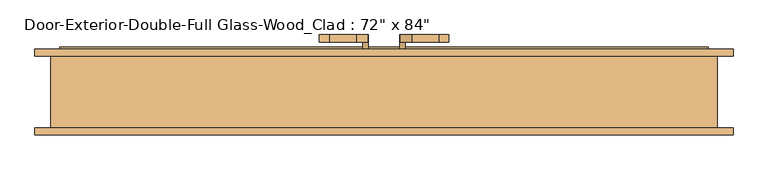
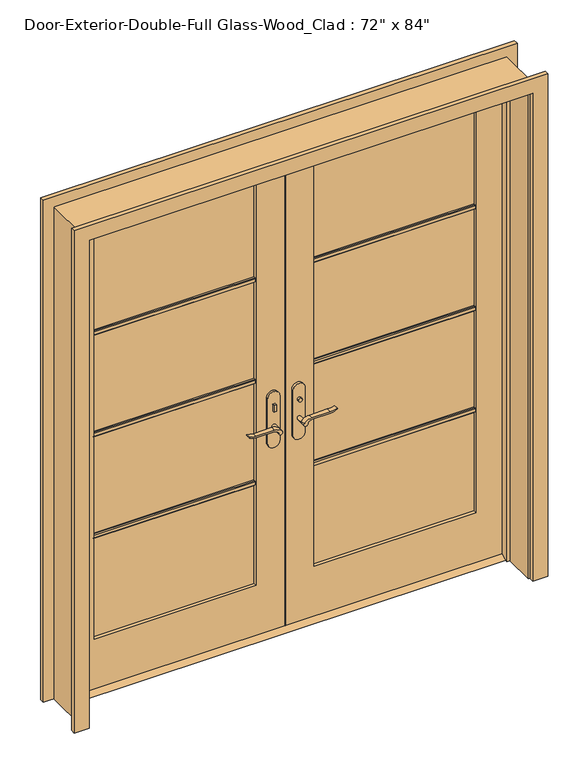
"""IFC4 building model written with IfcOpenShell, lengths in millimetres: door geometry."""

from ifc_helpers import new_model, si_unit, point, frame, frame_2d, origin, place, context, project, spatial, polyline, circle_curve, trimmed, segment, composite_curve, outline, extrude, faceted_brep, source, transform, mapped, element, save


def door_06d7e188(model_context):
    return source(origin(), model_context, "Body", "SolidModel", [
        extrude(outline(polyline([(63.5, 12.7), (98.425, 12.7), (123.825, 0.0), (38.1, 0.0), (63.5, 12.7)])), frame((-914.4, 0.0, 0.0), z_axis=(1.0, 0.0, 0.0), x_axis=(0.0, 1.0, 0.0)), (0.0, 0.0, 1.0), 1828.8),
        extrude(outline(polyline([(-47.4019111, 43.5), (-57.4019111, 43.5), (-57.4019111, 53.5), (-47.4019111, 53.5), (-47.4019111, 43.5)])), frame((0.0, 0.0, 981.9), z_axis=(0.0, 0.0, 1.0), x_axis=(1.0, 0.0, 0.0)), (0.0, 0.0, 1.0), 30.0),
        extrude(outline(composite_curve([segment(trimmed(circle_curve(frame_2d((996.9, -52.4019111)), 8.0), [point((996.9, -60.4019111))], [point((996.9, -44.4019111))], False, "CARTESIAN"), True, "CONTINUOUS"), segment(trimmed(circle_curve(frame_2d((996.9, -52.4019111)), 8.0), [point((996.9, -44.4019111))], [point((996.9, -60.4019111))], False, "CARTESIAN"), True, "CONTINUOUS")], self_intersect=False)), frame((0.0, 108.425, 0.0), z_axis=(0.0, 1.0, 0.0), x_axis=(0.0, 0.0, 1.0)), (0.0, 0.0, 1.0), 10.0),
        extrude(outline(composite_curve([segment(trimmed(circle_curve(frame_2d((897.1555521, -76.0694241)), 37.2832219), [point((919.0523287, -45.8937749))], [point((934.4, -77.7693445))], False, "CARTESIAN"), True, "CONTINUOUS"), segment(polyline([(934.4, -77.7693445), (934.4, -154.045502)]), True, "CONTINUOUS"), segment(trimmed(circle_curve(frame_2d((1017.6850638, -153.9791202)), 83.2850902), [point((934.4, -154.045502))], [point((939.4, -182.4019111))], True, "CARTESIAN"), True, "CONTINUOUS"), segment(polyline([(939.4, -182.4019111), (936.6135558, -182.4019111)]), True, "CONTINUOUS"), segment(trimmed(circle_curve(frame_2d((986.6709207, -150.4622499)), 59.3791355), [point((936.6135558, -182.4019111))], [point((927.4, -154.045502))], False, "CARTESIAN"), True, "CONTINUOUS"), segment(polyline([(927.4, -154.045502), (927.4, -77.7881013)]), True, "CONTINUOUS"), segment(trimmed(circle_curve(frame_2d((909.2738613, -77.7881013)), 18.1261387), [point((927.4, -77.7881013))], [point((914.4, -60.4019111))], True, "CARTESIAN"), True, "CONTINUOUS"), segment(trimmed(circle_curve(frame_2d((914.4, -52.4019111)), 8.0), [point((914.4, -60.4019111))], [point((919.0523287, -45.8937749))], False, "CARTESIAN"), True, "CONTINUOUS")], self_intersect=False)), frame((0.0, 3.5, 0.0), z_axis=(0.0, 1.0, 0.0), x_axis=(0.0, 0.0, 1.0)), (0.0, 0.0, 1.0), 20.0),
        extrude(outline(composite_curve([segment(trimmed(circle_curve(frame_2d((914.4, -52.4019111)), 8.0), [point((914.3999903, -60.4019111))], [point((919.0523287, -45.8937749))], False, "CARTESIAN"), True, "CONTINUOUS"), segment(trimmed(circle_curve(frame_2d((897.1555521, -76.0694241)), 37.2832219), [point((919.0523287, -45.8937749))], [point((934.4, -77.7693445))], False, "CARTESIAN"), True, "CONTINUOUS"), segment(polyline([(934.4, -77.7693445), (934.4, -154.045502)]), True, "CONTINUOUS"), segment(trimmed(circle_curve(frame_2d((1017.6850638, -153.9791202)), 83.2850902), [point((934.4, -154.045502))], [point((939.4, -182.4019111))], True, "CARTESIAN"), True, "CONTINUOUS"), segment(polyline([(939.4, -182.4019111), (936.6135558, -182.4019111)]), True, "CONTINUOUS"), segment(trimmed(circle_curve(frame_2d((986.6709207, -150.4622499)), 59.3791355), [point((936.6135558, -182.4019111))], [point((927.4, -154.045502))], False, "CARTESIAN"), True, "CONTINUOUS"), segment(polyline([(927.4, -154.045502), (927.4, -77.788099)]), True, "CONTINUOUS"), segment(trimmed(circle_curve(frame_2d((909.2738682, -77.788099)), 18.1261318), [point((927.4, -77.788099))], [point((914.3999903, -60.4019111))], True, "CARTESIAN"), True, "CONTINUOUS")], self_intersect=False)), frame((0.0, 138.425, 0.0), z_axis=(0.0, 1.0, 0.0), x_axis=(0.0, 0.0, 1.0)), (0.0, 0.0, 1.0), 20.0),
        extrude(outline(composite_curve([segment(trimmed(circle_curve(frame_2d((914.4, -52.4019111)), 8.0), [point((914.4, -60.4019111))], [point((914.4, -44.4019111))], False, "CARTESIAN"), True, "CONTINUOUS"), segment(trimmed(circle_curve(frame_2d((914.4, -52.4019111)), 8.0), [point((914.4, -44.4019111))], [point((914.4, -60.4019111))], False, "CARTESIAN"), True, "CONTINUOUS")], self_intersect=False)), frame((0.0, 23.5, 0.0), z_axis=(0.0, 1.0, 0.0), x_axis=(0.0, 0.0, 1.0)), (0.0, 0.0, 1.0), 30.0),
        extrude(outline(composite_curve([segment(trimmed(circle_curve(frame_2d((914.4, -52.4019111)), 8.0), [point((914.4, -60.4019111))], [point((914.4, -44.4019111))], False, "CARTESIAN"), True, "CONTINUOUS"), segment(trimmed(circle_curve(frame_2d((914.4, -52.4019111)), 8.0), [point((914.4, -44.4019111))], [point((914.4, -60.4019111))], False, "CARTESIAN"), True, "CONTINUOUS")], self_intersect=False)), frame((0.0, 108.425, 0.0), z_axis=(0.0, 1.0, 0.0), x_axis=(0.0, 0.0, 1.0)), (0.0, 0.0, 1.0), 30.0),
        extrude(outline(composite_curve([segment(polyline([(844.4, -27.4019111), (1039.4, -27.4019111)]), True, "CONTINUOUS"), segment(trimmed(circle_curve(frame_2d((1039.4, -52.4019111)), 25.0), [point((1039.4, -27.4019111))], [point((1039.4, -77.4019111))], False, "CARTESIAN"), True, "CONTINUOUS"), segment(polyline([(1039.4, -77.4019111), (844.4, -77.4019111)]), True, "CONTINUOUS"), segment(trimmed(circle_curve(frame_2d((844.4, -52.4019111)), 25.0), [point((844.4, -77.4019111))], [point((844.4, -27.4019111))], False, "CARTESIAN"), True, "CONTINUOUS")], self_intersect=False)), frame((0.0, 53.5, 0.0), z_axis=(0.0, 1.0, 0.0), x_axis=(0.0, 0.0, 1.0)), (0.0, 0.0, 1.0), 10.0),
        extrude(outline(composite_curve([segment(polyline([(844.4, -27.4019111), (1039.4, -27.4019111)]), True, "CONTINUOUS"), segment(trimmed(circle_curve(frame_2d((1039.4, -52.4019111)), 25.0), [point((1039.4, -27.4019111))], [point((1039.4, -77.4019111))], False, "CARTESIAN"), True, "CONTINUOUS"), segment(polyline([(1039.4, -77.4019111), (844.4, -77.4019111)]), True, "CONTINUOUS"), segment(trimmed(circle_curve(frame_2d((844.4, -52.4019111)), 25.0), [point((844.4, -77.4019111))], [point((844.4, -27.4019111))], False, "CARTESIAN"), True, "CONTINUOUS")], self_intersect=False)), frame((0.0, 98.425, 0.0), z_axis=(0.0, 1.0, 0.0), x_axis=(0.0, 0.0, 1.0)), (0.0, 0.0, 1.0), 10.0),
        extrude(outline(polyline([(47.3875, 118.425), (57.3875, 118.425), (57.3875, 108.425), (47.3875, 108.425), (47.3875, 118.425)])), frame((0.0, 0.0, 981.9), z_axis=(0.0, 0.0, 1.0), x_axis=(1.0, 0.0, 0.0)), (0.0, 0.0, 1.0), 30.0),
        extrude(outline(composite_curve([segment(trimmed(circle_curve(frame_2d((996.9, 52.3875)), 8.0), [point((996.9, 60.3875))], [point((996.9, 44.3875))], False, "CARTESIAN"), True, "CONTINUOUS"), segment(trimmed(circle_curve(frame_2d((996.9, 52.3875)), 8.0), [point((996.9, 44.3875))], [point((996.9, 60.3875))], False, "CARTESIAN"), True, "CONTINUOUS")], self_intersect=False)), frame((0.0, 43.5, 0.0), z_axis=(0.0, 1.0, 0.0), x_axis=(0.0, 0.0, 1.0)), (0.0, 0.0, 1.0), 10.0),
        extrude(outline(composite_curve([segment(trimmed(circle_curve(frame_2d((914.4, 52.3875)), 8.0), [point((919.0523287, 45.8793637))], [point((914.4, 60.3875))], False, "CARTESIAN"), True, "CONTINUOUS"), segment(trimmed(circle_curve(frame_2d((909.2738613, 77.7736901)), 18.1261387), [point((914.4, 60.3875))], [point((927.4, 77.7736901))], True, "CARTESIAN"), True, "CONTINUOUS"), segment(polyline([(927.4, 77.7736901), (927.4, 154.0310909)]), True, "CONTINUOUS"), segment(trimmed(circle_curve(frame_2d((986.6709207, 150.4478388)), 59.3791355), [point((927.4, 154.0310909))], [point((936.6135558, 182.3875))], False, "CARTESIAN"), True, "CONTINUOUS"), segment(polyline([(936.6135558, 182.3875), (939.4, 182.3875)]), True, "CONTINUOUS"), segment(trimmed(circle_curve(frame_2d((1017.6850638, 153.9647091)), 83.2850902), [point((939.4, 182.3875))], [point((934.4, 154.0310909))], True, "CARTESIAN"), True, "CONTINUOUS"), segment(polyline([(934.4, 154.0310909), (934.4, 77.7549333)]), True, "CONTINUOUS"), segment(trimmed(circle_curve(frame_2d((897.1555521, 76.0550129)), 37.2832219), [point((934.4, 77.7549333))], [point((919.0523287, 45.8793637))], False, "CARTESIAN"), True, "CONTINUOUS")], self_intersect=False)), frame((0.0, 138.425, 0.0), z_axis=(0.0, 1.0, 0.0), x_axis=(0.0, 0.0, 1.0)), (0.0, 0.0, 1.0), 20.0),
        extrude(outline(composite_curve([segment(trimmed(circle_curve(frame_2d((909.2738682, 77.7736878)), 18.1261318), [point((914.3999903, 60.3875))], [point((927.4, 77.7736878))], True, "CARTESIAN"), True, "CONTINUOUS"), segment(polyline([(927.4, 77.7736878), (927.4, 154.0310909)]), True, "CONTINUOUS"), segment(trimmed(circle_curve(frame_2d((986.6709207, 150.4478388)), 59.3791355), [point((927.4, 154.0310909))], [point((936.6135558, 182.3875))], False, "CARTESIAN"), True, "CONTINUOUS"), segment(polyline([(936.6135558, 182.3875), (939.4, 182.3875)]), True, "CONTINUOUS"), segment(trimmed(circle_curve(frame_2d((1017.6850638, 153.9647091)), 83.2850902), [point((939.4, 182.3875))], [point((934.4, 154.0310909))], True, "CARTESIAN"), True, "CONTINUOUS"), segment(polyline([(934.4, 154.0310909), (934.4, 77.7549333)]), True, "CONTINUOUS"), segment(trimmed(circle_curve(frame_2d((897.1555521, 76.0550129)), 37.2832219), [point((934.4, 77.7549333))], [point((919.0523287, 45.8793637))], False, "CARTESIAN"), True, "CONTINUOUS"), segment(trimmed(circle_curve(frame_2d((914.4, 52.3875)), 8.0), [point((919.0523287, 45.8793637))], [point((914.3999903, 60.3875))], False, "CARTESIAN"), True, "CONTINUOUS")], self_intersect=False)), frame((0.0, 3.5, 0.0), z_axis=(0.0, 1.0, 0.0), x_axis=(0.0, 0.0, 1.0)), (0.0, 0.0, 1.0), 20.0),
        extrude(outline(composite_curve([segment(trimmed(circle_curve(frame_2d((914.4, 52.3875)), 8.0), [point((914.4, 60.3875))], [point((914.4, 44.3875))], False, "CARTESIAN"), True, "CONTINUOUS"), segment(trimmed(circle_curve(frame_2d((914.4, 52.3875)), 8.0), [point((914.4, 44.3875))], [point((914.4, 60.3875))], False, "CARTESIAN"), True, "CONTINUOUS")], self_intersect=False)), frame((0.0, 108.425, 0.0), z_axis=(0.0, 1.0, 0.0), x_axis=(0.0, 0.0, 1.0)), (0.0, 0.0, 1.0), 30.0),
        extrude(outline(composite_curve([segment(trimmed(circle_curve(frame_2d((914.4, 52.3875)), 8.0), [point((914.4, 60.3875))], [point((914.4, 44.3875))], False, "CARTESIAN"), True, "CONTINUOUS"), segment(trimmed(circle_curve(frame_2d((914.4, 52.3875)), 8.0), [point((914.4, 44.3875))], [point((914.4, 60.3875))], False, "CARTESIAN"), True, "CONTINUOUS")], self_intersect=False)), frame((0.0, 23.5, 0.0), z_axis=(0.0, 1.0, 0.0), x_axis=(0.0, 0.0, 1.0)), (0.0, 0.0, 1.0), 30.0),
        extrude(outline(composite_curve([segment(trimmed(circle_curve(frame_2d((844.4, 52.3875)), 25.0), [point((844.4, 27.3875))], [point((844.4, 77.3875))], False, "CARTESIAN"), True, "CONTINUOUS"), segment(polyline([(844.4, 77.3875), (1039.4, 77.3875)]), True, "CONTINUOUS"), segment(trimmed(circle_curve(frame_2d((1039.4, 52.3875)), 25.0), [point((1039.4, 77.3875))], [point((1039.4, 27.3875))], False, "CARTESIAN"), True, "CONTINUOUS"), segment(polyline([(1039.4, 27.3875), (844.4, 27.3875)]), True, "CONTINUOUS")], self_intersect=False)), frame((0.0, 98.425, 0.0), z_axis=(0.0, 1.0, 0.0), x_axis=(0.0, 0.0, 1.0)), (0.0, 0.0, 1.0), 10.0),
        extrude(outline(composite_curve([segment(trimmed(circle_curve(frame_2d((844.4, 52.3875)), 25.0), [point((844.4, 27.3875))], [point((844.4, 77.3875))], False, "CARTESIAN"), True, "CONTINUOUS"), segment(polyline([(844.4, 77.3875), (1039.4, 77.3875)]), True, "CONTINUOUS"), segment(trimmed(circle_curve(frame_2d((1039.4, 52.3875)), 25.0), [point((1039.4, 77.3875))], [point((1039.4, 27.3875))], False, "CARTESIAN"), True, "CONTINUOUS"), segment(polyline([(1039.4, 27.3875), (844.4, 27.3875)]), True, "CONTINUOUS")], self_intersect=False)), frame((0.0, 53.5, 0.0), z_axis=(0.0, 1.0, 0.0), x_axis=(0.0, 0.0, 1.0)), (0.0, 0.0, 1.0), 10.0),
        extrude(outline(polyline([(77.47, 1578.371875), (77.47, 1559.321875), (71.12, 1559.321875), (67.945, 1562.496875), (67.945, 1575.196875), (71.12, 1578.371875), (77.47, 1578.371875)])), frame((120.65, 0.0, 0.0), z_axis=(1.0, 0.0, 0.0), x_axis=(0.0, 1.0, 0.0)), (0.0, 0.0, 1.0), 673.1),
        extrude(outline(polyline([(77.47, 1132.68125), (77.47, 1113.63125), (71.12, 1113.63125), (67.945, 1116.80625), (67.945, 1129.50625), (71.12, 1132.68125), (77.47, 1132.68125)])), frame((120.65, 0.0, 0.0), z_axis=(1.0, 0.0, 0.0), x_axis=(0.0, 1.0, 0.0)), (0.0, 0.0, 1.0), 673.1),
        extrude(outline(polyline([(77.47, 686.990625), (77.47, 667.940625), (71.12, 667.940625), (67.945, 671.115625), (67.945, 683.815625), (71.12, 686.990625), (77.47, 686.990625)])), frame((120.65, 0.0, 0.0), z_axis=(1.0, 0.0, 0.0), x_axis=(0.0, 1.0, 0.0)), (0.0, 0.0, 1.0), 673.1),
        extrude(outline(polyline([(84.455, 1578.371875), (90.805, 1578.371875), (93.98, 1575.196875), (93.98, 1562.496875), (90.805, 1559.321875), (84.455, 1559.321875), (84.455, 1578.371875)])), frame((-793.75, 0.0, 0.0), z_axis=(1.0, 0.0, 0.0), x_axis=(0.0, 1.0, 0.0)), (0.0, 0.0, 1.0), 673.1),
        extrude(outline(polyline([(84.455, 1132.68125), (90.805, 1132.68125), (93.98, 1129.50625), (93.98, 1116.80625), (90.805, 1113.63125), (84.455, 1113.63125), (84.455, 1132.68125)])), frame((-793.75, 0.0, 0.0), z_axis=(1.0, 0.0, 0.0), x_axis=(0.0, 1.0, 0.0)), (0.0, 0.0, 1.0), 673.1),
        extrude(outline(polyline([(84.455, 686.990625), (90.805, 686.990625), (93.98, 683.815625), (93.98, 671.115625), (90.805, 667.940625), (84.455, 667.940625), (84.455, 686.990625)])), frame((-793.75, 0.0, 0.0), z_axis=(1.0, 0.0, 0.0), x_axis=(0.0, 1.0, 0.0)), (0.0, 0.0, 1.0), 673.1),
        extrude(outline(polyline([(84.455, 1578.371875), (90.805, 1578.371875), (93.98, 1575.196875), (93.98, 1562.496875), (90.805, 1559.321875), (84.455, 1559.321875), (84.455, 1578.371875)])), frame((120.65, 0.0, 0.0), z_axis=(1.0, 0.0, 0.0), x_axis=(0.0, 1.0, 0.0)), (0.0, 0.0, 1.0), 673.1),
        extrude(outline(polyline([(84.455, 1132.68125), (90.805, 1132.68125), (93.98, 1129.50625), (93.98, 1116.80625), (90.805, 1113.63125), (84.455, 1113.63125), (84.455, 1132.68125)])), frame((120.65, 0.0, 0.0), z_axis=(1.0, 0.0, 0.0), x_axis=(0.0, 1.0, 0.0)), (0.0, 0.0, 1.0), 673.1),
        extrude(outline(polyline([(84.455, 686.990625), (90.805, 686.990625), (93.98, 683.815625), (93.98, 671.115625), (90.805, 667.940625), (84.455, 667.940625), (84.455, 686.990625)])), frame((120.65, 0.0, 0.0), z_axis=(1.0, 0.0, 0.0), x_axis=(0.0, 1.0, 0.0)), (0.0, 0.0, 1.0), 673.1),
        extrude(outline(polyline([(77.47, 1578.371875), (77.47, 1559.321875), (71.12, 1559.321875), (67.945, 1562.496875), (67.945, 1575.196875), (71.12, 1578.371875), (77.47, 1578.371875)])), frame((-793.75, 0.0, 0.0), z_axis=(1.0, 0.0, 0.0), x_axis=(0.0, 1.0, 0.0)), (0.0, 0.0, 1.0), 673.1),
        extrude(outline(polyline([(77.47, 1132.68125), (77.47, 1113.63125), (71.12, 1113.63125), (67.945, 1116.80625), (67.945, 1129.50625), (71.12, 1132.68125), (77.47, 1132.68125)])), frame((-793.75, 0.0, 0.0), z_axis=(1.0, 0.0, 0.0), x_axis=(0.0, 1.0, 0.0)), (0.0, 0.0, 1.0), 673.1),
        extrude(outline(polyline([(77.47, 686.990625), (77.47, 667.940625), (71.12, 667.940625), (67.945, 671.115625), (67.945, 683.815625), (71.12, 686.990625), (77.47, 686.990625)])), frame((-793.75, 0.0, 0.0), z_axis=(1.0, 0.0, 0.0), x_axis=(0.0, 1.0, 0.0)), (0.0, 0.0, 1.0), 673.1),
        extrude(outline(polyline([(0.0, 920.75), (0.0, 984.25), (2203.45, 984.25), (2203.45, -984.25), (0.0, -984.25), (0.0, -920.75), (2139.95, -920.75), (2139.95, 920.75), (0.0, 920.75)])), frame((0.0, 98.425, 0.0), z_axis=(0.0, 1.0, 0.0), x_axis=(0.0, 0.0, 1.0)), (0.0, 0.0, 1.0), 19.05),
        extrude(outline(polyline([(0.0, 920.75), (0.0, 984.25), (2203.45, 984.25), (2203.45, -984.25), (0.0, -984.25), (0.0, -920.75), (2139.95, -920.75), (2139.95, 920.75), (0.0, 920.75)])), frame((0.0, -123.825, 0.0), z_axis=(0.0, 1.0, 0.0), x_axis=(0.0, 0.0, 1.0)), (0.0, 0.0, 1.0), 19.05),
        extrude(outline(polyline([(12.7, 914.4), (2133.6, 914.4), (2133.6, 1.5875), (12.7, 1.5875), (12.7, 914.4)]), holes=[polyline([(2014.5375, 120.65), (2014.5375, 793.75), (231.775, 793.75), (231.775, 120.65), (2014.5375, 120.65)])]), frame((0.0, 63.5, 0.0), z_axis=(0.0, 1.0, 0.0), x_axis=(0.0, 0.0, 1.0)), (0.0, 0.0, 1.0), 34.925),
        extrude(outline(polyline([(2133.6, -914.4), (12.7, -914.4), (12.7, -1.6019111), (2133.6, -1.6019111), (2133.6, -914.4)]), holes=[polyline([(231.775, -793.75), (2014.5375, -793.75), (2014.5375, -120.65), (231.775, -120.65), (231.775, -793.75)])]), frame((0.0, 63.5, 0.0), z_axis=(0.0, 1.0, 0.0), x_axis=(0.0, 0.0, 1.0)), (0.0, 0.0, 1.0), 34.925),
        faceted_brep([(939.8, 98.425, 0.0), (939.8, -104.775, 0.0), (914.4, -104.775, 0.0), (914.4, 28.575, 0.0), (901.7, 28.575, 0.0), (901.7, 63.5, 0.0), (914.4, 63.5, 0.0), (914.4, 98.425, 0.0), (939.8, 98.425, 2159.0), (939.8, -104.775, 2159.0), (-939.8, -104.775, 2159.0), (-939.8, -104.775, 0.0), (-914.4, -104.775, 0.0), (-914.4, -104.775, 2133.6), (914.4, -104.775, 2133.6), (914.4, 28.575, 2133.6), (-914.4, 28.575, 2133.6), (-914.4, 28.575, 0.0), (-901.7, 28.575, 0.0), (-901.7, 28.575, 2120.9), (901.7, 28.575, 2120.9), (901.7, 63.5, 2120.9), (1.5875, 63.5, 2120.9), (-1.6019111, 63.5, 2120.9), (-901.7, 63.5, 2120.9), (-901.7, 63.5, 0.0), (-914.4, 63.5, 0.0), (-914.4, 63.5, 2133.6), (-1.6019111, 63.5, 2133.6), (1.5875, 63.5, 2133.6), (914.4, 63.5, 2133.6), (914.4, 98.425, 2133.6), (1.5875, 98.425, 2133.6), (-1.6019111, 98.425, 2133.6), (-914.4, 98.425, 2133.6), (-914.4, 98.425, 0.0), (-939.8, 98.425, 0.0), (-939.8, 98.425, 2159.0)], [[[0, 1, 2, 3, 4, 5, 6, 7]], [[1, 0, 8, 9]], [[2, 1, 9, 10, 11, 12, 13, 14]], [[3, 2, 14, 15]], [[4, 3, 15, 16, 17, 18, 19, 20]], [[5, 4, 20, 21]], [[6, 5, 21, 22, 23, 24, 25, 26, 27, 28, 29, 30]], [[7, 6, 30, 31]], [[0, 7, 31, 32, 33, 34, 35, 36, 37, 8]], [[9, 8, 37, 10]], [[14, 13, 16, 15]], [[20, 19, 24, 23, 22, 21]], [[31, 30, 29, 28, 27, 34, 33, 32]], [[12, 11, 36, 35, 26, 25, 18, 17]], [[11, 10, 37, 36]], [[13, 12, 17, 16]], [[19, 18, 25, 24]], [[27, 26, 35, 34]]]),
        extrude(outline(polyline([(793.75, 77.47), (120.65, 77.47), (120.65, 84.455), (793.75, 84.455), (793.75, 77.47)])), frame((0.0, 0.0, 231.775), z_axis=(0.0, 0.0, 1.0), x_axis=(1.0, 0.0, 0.0)), (0.0, 0.0, 1.0), 1782.7625),
        extrude(outline(polyline([(-120.65, 77.47), (-793.75, 77.47), (-793.75, 84.455), (-120.65, 84.455), (-120.65, 77.47)])), frame((0.0, 0.0, 231.775), z_axis=(0.0, 0.0, 1.0), x_axis=(1.0, 0.0, 0.0)), (0.0, 0.0, 1.0), 1782.7625),
    ])


if __name__ == "__main__":
    model = new_model("IFC4")
    model_context = context("Model", 3, world=origin())
    ifc_project = project(units=[si_unit("LENGTHUNIT", "METRE", prefix="MILLI")], contexts=[model_context])
    site = spatial("IfcSite", under=ifc_project)
    building = spatial("IfcBuilding", under=site)
    placement = place(None, origin())
    door_shape = door_06d7e188(model_context)
    element("IfcDoor", 1, ObjectType="Door-Exterior-Double-Full Glass-Wood_Clad : 72\" x 84\"", at=placement, inside=building, context=model_context, shape_type="MappedRepresentation", body=[
        mapped(door_shape, transform((0.0, 0.0, 0.0), x_axis=(1.0, 0.0, 0.0), y_axis=(0.0, 1.0, 0.0), z_axis=(0.0, 0.0, 1.0))),
    ])
    save(model, "model.ifc")

# Revit data of these elements
# Type "Door-Exterior-Double-Full Glass-Wood_Clad : 72\" x 84\""
#   Type Mark = "8"
#   Assembly Code = "B2030100"
#   Analytic Construction = "French door, wood frame with double glass"
#   Top Rail = 0' - 4 11/16"
#   Threshold Offset [instance default] = 0' - 0 1/2"
#   Thickness = 0' - 1 3/8"
#   Thermal Resistance (R) = 1.9158 (h·ft²·°F)/BTU
#   Swing Angle [instance default] = 90.00°
#   Stiles = 0' - 4 3/4"
#   Rough Width = 6' - 2"
#   Rough Height = 7' - 1"
#   Panel Width = 3' - 0"
#   Door Offset [instance default] = 0' - 0"
#   Height = 7' - 0"
#   Width = 6' - 0"
#   Heat Transfer Coefficient (U) = 0.5220 BTU/(h·ft²·°F)
#   Bottom Rail = 0' - 9 1/8"
#   Exterior Trim [instance default] = yes
#   Threshold [instance default] = yes
#   Show Grill [instance default] = yes
#   Function = 1
#   Trim Material = Cherry
#   Threshold Material = Cherry
#   Panel Material = Cherry
#   Glazing = Glass
#   Frame Material = Cherry
#   Door Handle Material = Aluminum
#   Visual Light Transmittance = 0
#   Solar Heat Gain Coefficient = 0
#   Wall Closure = (empty or 0)
#   Construction Type = (empty or 0)
# Element 1 (IfcDoor, "Door-Exterior-Double-Full Glass-Wood_Clad : 72\" x 84\"")
#   Materials on its faces: "Cherry", "Aluminum", "Glass"
# Materials
#   "Cherry": class "Wood", colour RGB 226 177 128, transparency 0, Description = "Prunus Serotina", Cost = 0
#   "Glass": class "Glass", colour RGB 0 128 192, transparency 0.75, Description = "Soda Lime Glass", Cost = 0
#   "Aluminum": class "Metal", colour RGB 247 247 247, transparency 0, Description = "Aluminum 6061", Cost = 0
